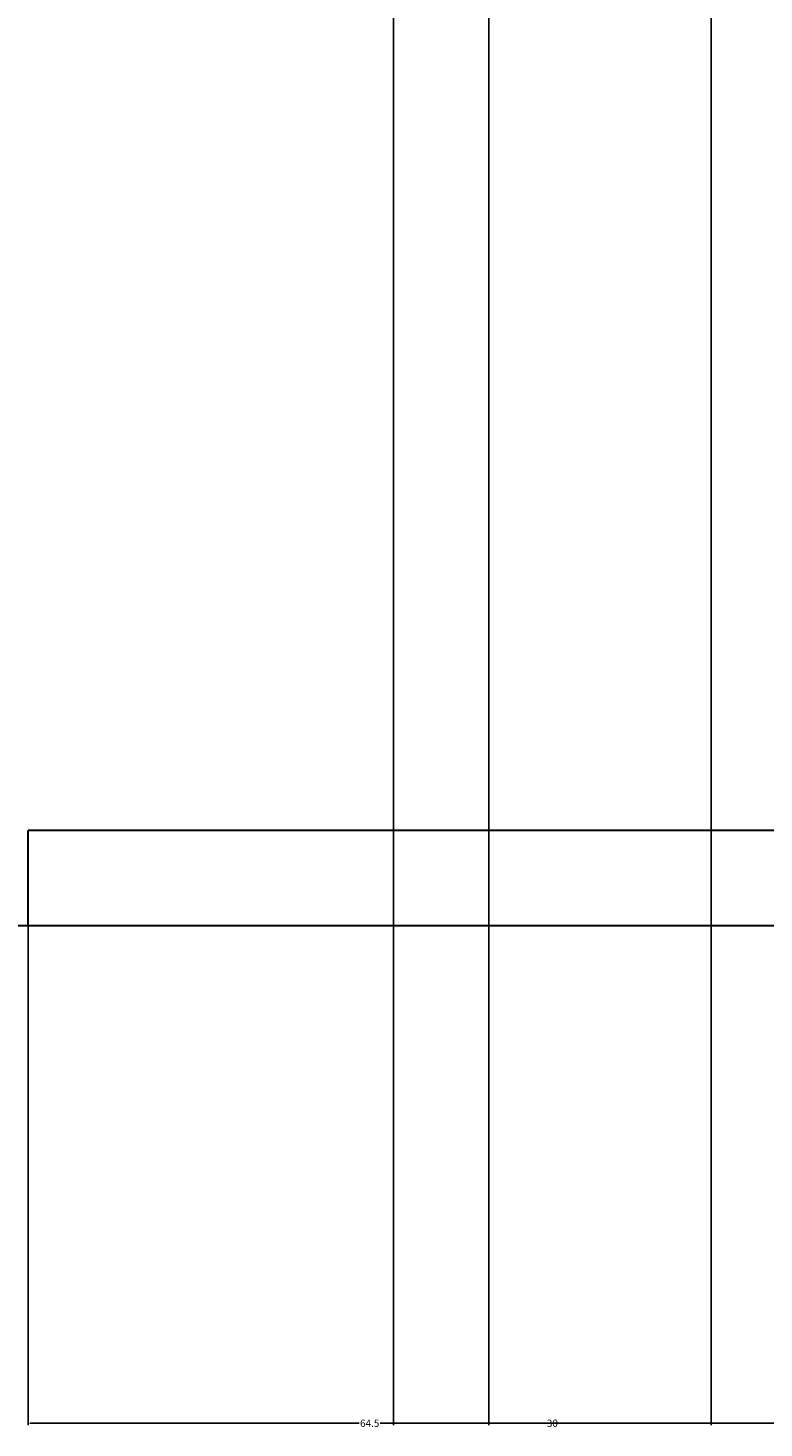
# Model space of a CAD drawing. Units: inches. Extents: x 867 to 1667, y -234 to 788.
# Tile 3 of 42: x 1006 to 1076, y -234 to -102. Entities that reach past the tile are written whole.
import ezdxf

# ---------------------------------------------------------------- set-up
doc = ezdxf.new("R2010")
doc.units = ezdxf.units.IN
doc.header["$MEASUREMENT"] = 0
doc.layers.add('A-ANNO-DIMS', color=2, linetype='Continuous', lineweight=18)
doc.layers.add('A-WALL-SITE', color=8, linetype='Continuous', lineweight=30)
doc.styles.get("Standard").update_dxf_attribs({"font": 'arial.ttf'})
doc.dimstyles.get("Standard").update_dxf_attribs({"dimtxt": 0.6875, "dimasz": 0.18, "dimexe": 0.18, "dimexo": 0.0625, "dimgap": 0.09, "dimtad": 0, "dimdec": 4, "dimzin": 0, "dimdsep": 46, "dimlunit": 4, "dimtxsty": 'Standard', "dimcen": 0.09, "dimadec": 0, "dimazin": 0, "dimtfac": 1, "dimtdec": 4, "dimtofl": 0, "dimtmove": 0, "dimatfit": 3, "dimfxl": 1, "dimtolj": 1, "dimtzin": 0, "dimarcsym": 0})

# ---------------------------------------------------------------- blocks, each defined once
blk = doc.blocks.new('*D25')
at = {"layer": 'A-ANNO-DIMS', "color": 0, "lineweight": -2, "transparency": 16777216}
for p, q in [((1070.89, -55.97), (1070.89, -233.54)), ((1006.39, -177.47), (1006.39, -233.54)), ((1006.57, -233.36), (1037.65, -233.36)), ((1070.71, -233.36), (1039.62, -233.36))]:
    blk.add_line(p, q, dxfattribs=at)
at = {"layer": 'A-ANNO-DIMS', "color": 0, "transparency": 16777216}
for points in [[(1006.57, -233.33), (1006.57, -233.39), (1006.39, -233.36)], [(1070.71, -233.33), (1070.71, -233.39), (1070.89, -233.36)]]:
    blk.add_solid(points, dxfattribs=at)
at = {"layer": 'Defpoints', "color": 0, "transparency": 16777216}
for p in [(1070.89, -55.91), (1006.39, -177.41), (1070.89, -233.36)]:
    blk.add_point(p, dxfattribs=at)
at = {"layer": 'A-ANNO-DIMS', "color": 0, "transparency": 16777216, "insert": (1038.64, -233.36), "char_height": 0.688, "attachment_point": 5}
blk.add_mtext('\\A1;64.5', dxfattribs=at)
blk = doc.blocks.new('*D27')
at = {"layer": 'A-ANNO-DIMS', "color": 0, "lineweight": -2, "transparency": 16777216}
for p, q in [((1070.89, -55.97), (1070.89, -233.54)), ((1525.26, -186.47), (1525.26, -233.54)), ((1071.07, -233.36), (1296.81, -233.36)), ((1525.08, -233.36), (1299.34, -233.36))]:
    blk.add_line(p, q, dxfattribs=at)
at = {"layer": 'A-ANNO-DIMS', "color": 0, "transparency": 16777216}
for points in [[(1071.07, -233.33), (1071.07, -233.39), (1070.89, -233.36)], [(1525.08, -233.33), (1525.08, -233.39), (1525.26, -233.36)]]:
    blk.add_solid(points, dxfattribs=at)
at = {"layer": 'Defpoints', "color": 0, "transparency": 16777216}
for p in [(1070.89, -55.91), (1525.26, -186.41), (1525.26, -233.36)]:
    blk.add_point(p, dxfattribs=at)
at = {"layer": 'A-ANNO-DIMS', "color": 0, "transparency": 16777216, "insert": (1298.08, -233.36), "char_height": 0.688, "attachment_point": 5}
blk.add_mtext('\\A1;454.4', dxfattribs=at)
blk = doc.blocks.new('*D37')
at = {"layer": 'A-ANNO-DIMS', "color": 0, "lineweight": -2, "transparency": 16777216}
for p, q in [((1049.89, 257.55), (1049.89, -233.54)), ((1196.89, 257.55), (1196.89, -233.54)), ((1050.07, -233.36), (1122.57, -233.36)), ((1196.71, -233.36), (1124.2, -233.36))]:
    blk.add_line(p, q, dxfattribs=at)
at = {"layer": 'A-ANNO-DIMS', "color": 0, "transparency": 16777216}
for points in [[(1050.07, -233.33), (1050.07, -233.39), (1049.89, -233.36)], [(1196.71, -233.33), (1196.71, -233.39), (1196.89, -233.36)]]:
    blk.add_solid(points, dxfattribs=at)
at = {"layer": 'Defpoints', "color": 0, "transparency": 16777216}
for p in [(1049.89, 257.62), (1196.89, 257.62), (1196.89, -233.36)]:
    blk.add_point(p, dxfattribs=at)
at = {"layer": 'A-ANNO-DIMS', "color": 0, "transparency": 16777216, "insert": (1123.39, -233.36), "char_height": 0.688, "attachment_point": 5}
blk.add_mtext('\\A1;147', dxfattribs=at)
blk = doc.blocks.new('*D49')
at = {"layer": 'A-ANNO-DIMS', "color": 0, "lineweight": -2, "transparency": 16777216}
for p, q in [((1070.89, -55.97), (1070.89, -233.54)), ((1211.89, -55.97), (1211.89, -233.54)), ((1071.07, -233.36), (1140.64, -233.36)), ((1211.71, -233.36), (1142.14, -233.36))]:
    blk.add_line(p, q, dxfattribs=at)
at = {"layer": 'A-ANNO-DIMS', "color": 0, "transparency": 16777216}
for points in [[(1071.07, -233.33), (1071.07, -233.39), (1070.89, -233.36)], [(1211.71, -233.33), (1211.71, -233.39), (1211.89, -233.36)]]:
    blk.add_solid(points, dxfattribs=at)
at = {"layer": 'Defpoints', "color": 0, "transparency": 16777216}
for p in [(1070.89, -55.91), (1211.89, -55.91), (1211.89, -233.36)]:
    blk.add_point(p, dxfattribs=at)
at = {"layer": 'A-ANNO-DIMS', "color": 0, "transparency": 16777216, "insert": (1141.39, -233.36), "char_height": 0.688, "attachment_point": 5}
blk.add_mtext('\\A1;141', dxfattribs=at)
blk = doc.blocks.new('*D63')
at = {"layer": 'A-ANNO-DIMS', "color": 0, "lineweight": -2, "transparency": 16777216}
for p, q in [((1040.89, 257.55), (1040.89, -233.54)), ((1070.89, 221.55), (1070.89, -233.54)), ((1041.07, -233.36), (1055.31, -233.36)), ((1070.71, -233.36), (1056.47, -233.36))]:
    blk.add_line(p, q, dxfattribs=at)
at = {"layer": 'A-ANNO-DIMS', "color": 0, "transparency": 16777216}
for points in [[(1041.07, -233.33), (1041.07, -233.39), (1040.89, -233.36)], [(1070.71, -233.33), (1070.71, -233.39), (1070.89, -233.36)]]:
    blk.add_solid(points, dxfattribs=at)
at = {"layer": 'Defpoints', "color": 0, "transparency": 16777216}
for p in [(1040.89, 257.62), (1070.89, 221.62), (1070.89, -233.36)]:
    blk.add_point(p, dxfattribs=at)
at = {"layer": 'A-ANNO-DIMS', "color": 0, "transparency": 16777216, "insert": (1055.89, -233.36), "char_height": 0.688, "attachment_point": 5}
blk.add_mtext('\\A1;30', dxfattribs=at)

msp = doc.modelspace()

# ---------------------------------------------------------------- linework, layer by layer
at = {"layer": 'A-WALL-SITE'}
for p, q in [((1006.3882, -186.4081), (1006.3882, -177.4081)), ((1526.8389, -177.4081), (1006.3882, -177.4081)), ((1619.8866, -186.4081), (914.8866, -186.4081))]:
    msp.add_line(p, q, dxfattribs=at)

# ---------------------------------------------------------------- dimensions: what is measured, and where the dimension line sits
at = {"layer": 'A-ANNO-DIMS'}
for base, p1, p2, override, picture, middle in [((1070.8866, -233.3581), (1040.8866, 257.617), (1070.8866, 221.617), {"dimdec": 0, "dimlfac": 1, "dimrnd": 0, "dimzin": 0, "dimdsep": 46, "dimlunit": 2}, '*D63', (1055.8866, -233.3581)), ((1196.8866, -233.3581), (1049.8866, 257.617), (1196.8866, 257.617), {"dimdec": 0, "dimlfac": 1, "dimrnd": 0, "dimzin": 0, "dimdsep": 46, "dimlunit": 2}, '*D37', (1123.3866, -233.3581)), ((1070.8866, -233.3581), (1006.3882, -177.4081), (1070.8866, -55.9081), {"dimdec": 1, "dimlfac": 1, "dimrnd": 0, "dimzin": 0, "dimdsep": 46, "dimlunit": 2}, '*D25', (1038.6374, -233.3581)), ((1525.2648, -233.3581), (1070.8866, -55.9081), (1525.2648, -186.4081), {"dimdec": 1, "dimlfac": 1, "dimrnd": 0, "dimzin": 0, "dimdsep": 46, "dimlunit": 2}, '*D27', (1298.0757, -233.3581)), ((1211.8866, -233.3581), (1070.8866, -55.9081), (1211.8866, -55.9081), {"dimdec": 0, "dimlfac": 1, "dimrnd": 0, "dimzin": 0, "dimdsep": 46, "dimlunit": 2}, '*D49', (1141.3866, -233.3581))]:
    dim = msp.add_linear_dim(base=base, p1=p1, p2=p2, dimstyle='Standard', override=override, dxfattribs=at)
    dim.commit()
    dim.dimension.update_dxf_attribs({"geometry": picture, "text_midpoint": middle})

doc.saveas('drawing.dxf')
